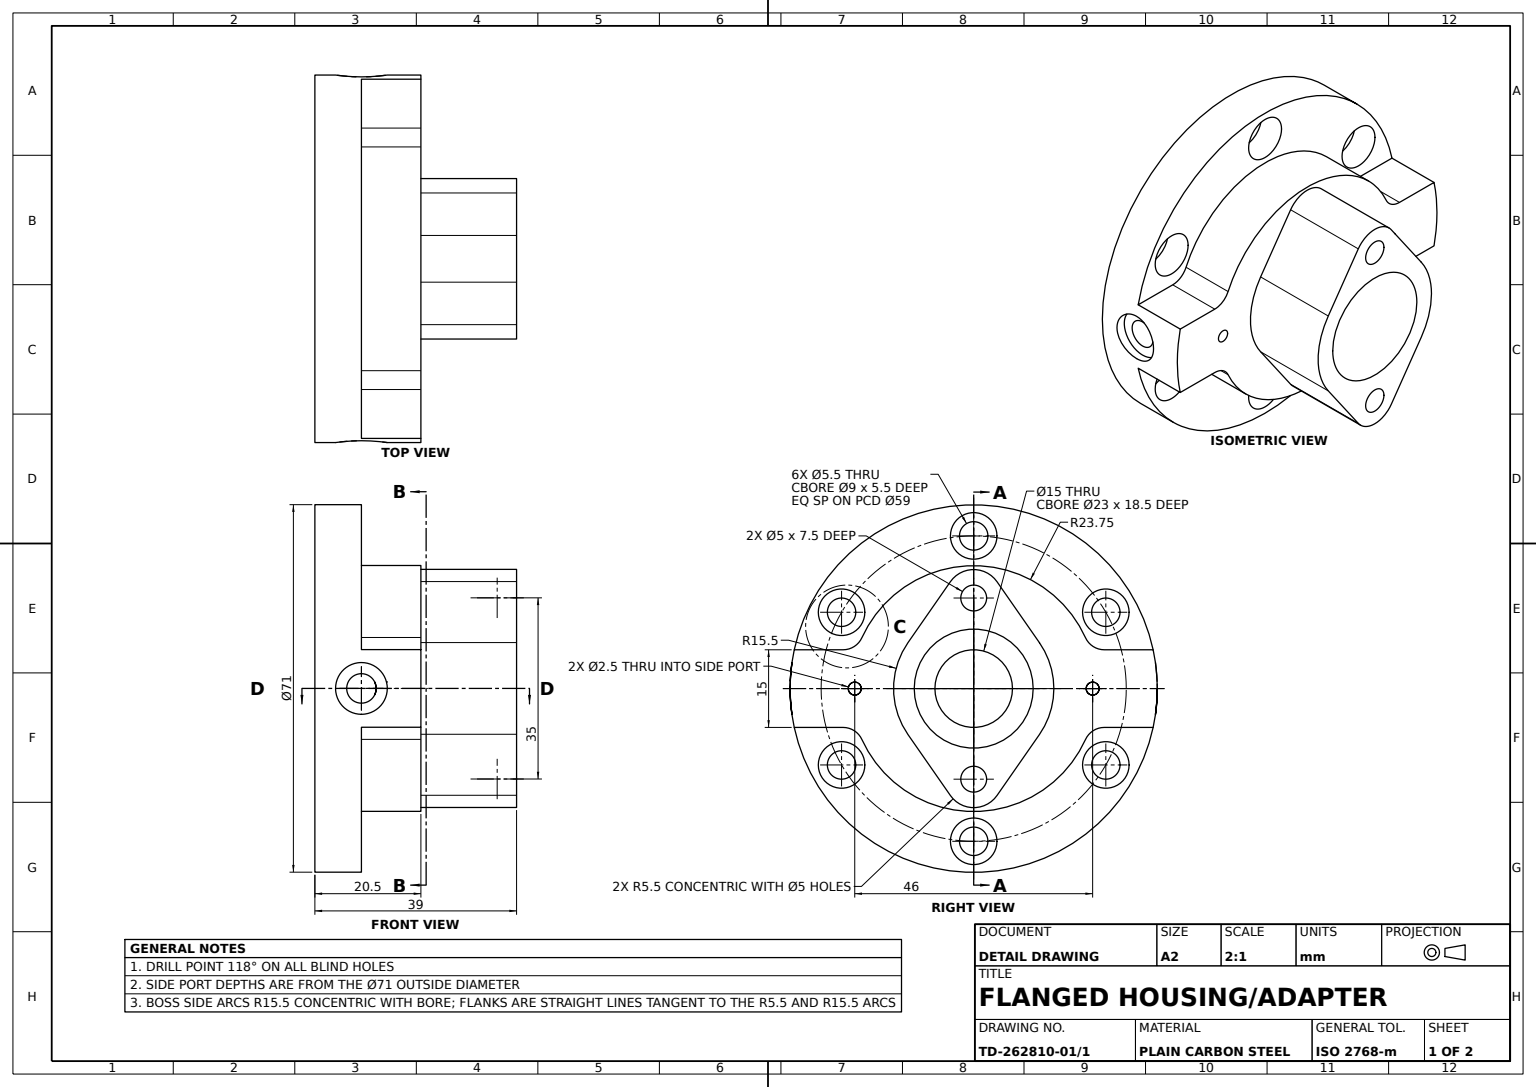
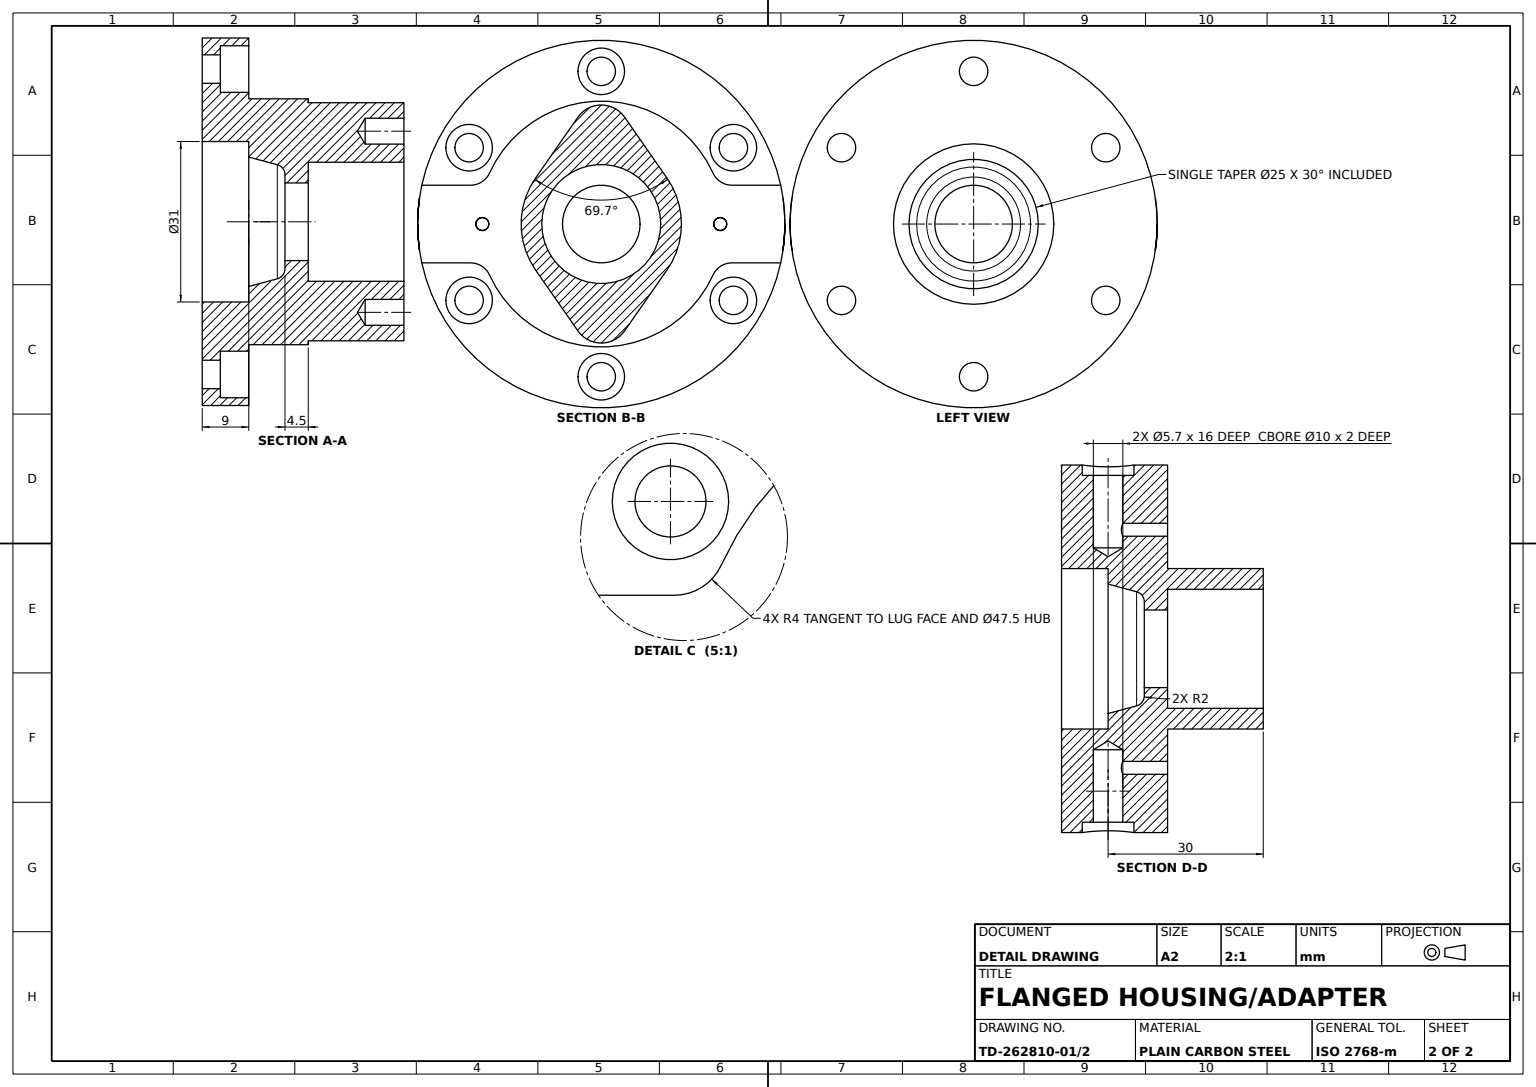
SolidWorks part; units mm, degrees
material "Plain Carbon Steel"
ref_plane "Front Plane" through (0, 0, 0) normal (0, 0, 1) x (1, 0, 0)
ref_plane "Top Plane" through (0, 0, 0) normal (0, 1, 0) x (1, 0, 0)
ref_plane "Right Plane" through (0, 0, 0) normal (1, 0, 0) x (0, 0, -1)
sketch "Flange Body Profile" plane through (0, 0, 0) normal (1, 0, 0) x (0, 0, -1)
  line L0 (0, 0) -> (0, 26.5052) construction
  line L1 (15.5, 0) -> (15.5, 9)
  line L2 (15.5, 9) -> (12.5, 9)
  line L3 (12.5, 9) -> (10.6244, 16)
  line L4 (10.6244, 16) -> (7.5, 16)
  line L5 (7.5, 16) -> (7.5, 20.5)
  line L6 (7.5, 20.5) -> (11.5, 20.5)
  line L7 (11.5, 20.5) -> (11.5, 39)
  line L8 (11.5, 39) -> (15.5, 39)
  line L9 (15.5, 39) -> (15.5, 9)
  line L10 (15.5, 9) -> (35.5, 9)
  line L11 (35.5, 9) -> (35.5, 0)
  line L12 (35.5, 0) -> (15.5, 0)
  dimension "D1" = 9
  dimension "D2" = 23
  dimension "D3" = 31
  dimension "D4" = 71
  dimension "D5" = 31
  dimension "D6" = 25
  dimension "D7" = 15
  dimension "D8" = 16
  dimension "D9" = 20.5
  dimension "D10" = 39
  dimension "D11" = 15
revolve "Flange Body" add sketch "Flange Body Profile" angle 360 about L0
sketch "Side Lug Profile" plane through (0, 39, 0) normal (0, 1, 0) x (1, 0, 0)
  line L0 (-17.5, 0) -> (17.5, 0) construction
  line L1 (-20.6429, 4.5136) -> (-8.8571, 12.7201)
  line L2 (20.6429, 4.5136) -> (8.8571, 12.7201)
  line L3 (20.6429, -4.5136) -> (8.8571, -12.7201)
  line L4 (-20.6429, -4.5136) -> (-8.8571, -12.7201)
  circle A0 centre (0, 0) radius 15.5 construction
  circle A1 centre (0, 0) radius 7.5 construction
  arc A2 (-8.8571, -12.7201) -> (8.8571, -12.7201) centre (0, 0) ccw
  circle A3 centre (0, 0) radius 7.5
  arc A4 (20.6429, -4.5136) -> (20.6429, 4.5136) centre (17.5, 0) ccw
  arc A5 (-20.6429, 4.5136) -> (-20.6429, -4.5136) centre (-17.5, 0) ccw
  arc A7 (8.8571, 12.7201) -> (-8.8571, 12.7201) centre (0, 0) ccw
  point P9 (0, 0)
  point P10 (0, 0)
  dimension "D2" = 11
  dimension "D1" = 35
extrude "Side Lugs" add sketch "Side Lug Profile" against normal blind 18.5
sketch "Oval Boss Profile" plane through (0, 9, 0) normal (0, 1, 0) x (1, 0, 0)
  line L0 (0, 35.5) -> (0, -35.5) construction
  line L1 (7.5, -34.6987) -> (7.5, -22.5347)
  line L2 (-7.5, -34.6987) -> (-7.5, -22.5347)
  line L3 (0, 0) -> (20.8022, 0) construction
  line L4 (7.5, 34.6987) -> (7.5, 22.5347)
  line L5 (-7.5, 34.6987) -> (-7.5, 22.5347)
  arc A0 (7.5, -22.5347) -> (7.5, 22.5347) centre (0, 0) ccw
  circle A1 centre (0, 0) radius 35.5 construction
  arc A2 (-7.5, -34.6987) -> (7.5, -34.6987) centre (0, 0) ccw
  arc A3 (-7.5, 34.6987) -> (7.5, 34.6987) centre (0, 0) cw
  arc A4 (-7.5, 22.5347) -> (-7.5, -22.5347) centre (0, 0) ccw
  dimension "D1" = 47.5
  dimension "D2" = 15
extrude "Oval Mounting Boss" add sketch "Oval Boss Profile" along normal up to surface (11.5 mm away) up to face at (17, 20.5, 0)
fillet "Boss Edge Fillet R4" radius 4 4 edges at (7.5, 14.75, -22.5347) (-7.5, 14.75, -22.5347) (-7.5, 14.75, 22.5347) (7.5, 14.75, 22.5347)
hole_wizard "Flange Holes 6x C'bore Ø5.5" positions "Sketch7" profile "Sketch8" legacy
sketch "Sketch7" plane through (0, 9, 0) normal (0, 1, 0) x (1, 0, 0)
  circle A0 centre (0, 0) radius 29.5 construction
  point P5 (-29.5, 0)
  point P11 (-14.75, 25.5477)
  point P12 (14.75, 25.5477)
  point P13 (29.5, 0)
  point P14 (14.75, -25.5477)
  point P15 (-14.75, -25.5477)
  dimension "D1" = 59
  dimension "D2" = 6
sketch "Sketch8" plane through (-14.75, 9, 25.5477) normal (1, 0, 0) x (0, 0, 1)
  line L0 (0, 0) -> (0, 9)
  line L1 (0, 9) -> (2.75, 9)
  line L2 (2.75, 9) -> (2.75, 5.5)
  line L3 (2.75, 5.5) -> (4.5, 5.5)
  line L4 (4.5, 5.5) -> (4.5, 0)
  line L5 (4.5, 0) -> (0, 0)
  line L6 (0, 110) -> (0, -10) construction
  dimension "Diameter" = 5.5
  dimension "Depth" = 9
  dimension "C-Bore Diameter" = 9
  dimension "C-Bore Depth" = 5.5
hole_wizard "Side Port C'bore Ø5.7" positions "3DSketch4" profile "Sketch13" legacy
sketch3d "3DSketch4"
  point P0 (0, 9, 35.5)
  point P9 (0, 9, -35.5)
sketch "Sketch13" plane through (0, 9, 35.5) normal (1, 0, 0) x (0, -1, 0)
  line L0 (0, 0) -> (0, 17.7125)
  line L1 (0, 17.7125) -> (2.85, 16)
  line L2 (2.85, 16) -> (2.85, 2)
  line L3 (2.85, 2) -> (5, 2)
  line L4 (5, 0) -> (0, 0)
  line L5 (0, -11.3109) -> (0, 121.1557) construction
  line L6 (0, 17.7125) -> (-2.85, 16) construction
  line L7 (5, 2) -> (5, 0)
  dimension "Depth" = 16
  dimension "Drill Angle" = 118
  dimension "Diameter" = 5.7
  dimension "C-Bore Diameter" = 10
  dimension "C-Bore Depth" = 2
sketch "Relief Cut Profile" plane through (0, 20.5, 0) normal (0, 1, 0) x (1, 0, 0)
  line L0 (0, 23) -> (0, -23) construction
  circle A0 centre (0, 23) radius 1.25
  circle A1 centre (0, -23) radius 1.25
  point P4 (0, 0)
  dimension "D2" = 2.5
  dimension "D1" = 46
extrude "Relief Cut" cut sketch "Relief Cut Profile" against normal up to next
hole_wizard "Lug Drill Holes Ø5" positions "Sketch15" profile "Sketch16" legacy
sketch "Sketch15" plane through (0, 39, 0) normal (0, 1, 0) x (1, 0, 0)
  point P0 (-17.5, 0)
  point P3 (17.5, 0)
sketch "Sketch16" plane through (-17.5, 39, 0) normal (1, 0, 0) x (0, 0, 1)
  line L0 (0, 0) -> (0, 9.0022)
  line L1 (0, 9.0022) -> (2.5, 7.5)
  line L2 (2.5, 7.5) -> (2.5, 0)
  line L4 (2.5, 0) -> (0, 0)
  line L6 (0, 9.0022) -> (-2.5, 7.5) construction
  line L7 (0, -4.2442) -> (0, 117.3081) construction
  dimension "Diameter" = 5
  dimension "Depth" = 7.5
  dimension "Drill Angle" = 118
sketch "Central Bore Profile" plane through (0, 0, 0) normal (1, 0, 0) x (0, 0, -1)
  line L0 (0, 0) -> (0, 26.5052) construction
  line L2 (21.6146, 9) -> (-21.6146, 9) construction
  line L4 (10.6244, 16) -> (7.5, 16) construction
  line L5 (12.5, 9) -> (10.6244, 16) construction
  line L6 (0, 0) -> (0, 39) construction
  line L7 (11.5, 20.5) -> (11.5, 39) construction
  line L8 (12.5, 9) -> (0, 9)
  line L10 (10.6244, 16) -> (7.5, 16)
  line L11 (12.5, 9) -> (10.6244, 16)
  line L14 (7.5, 20.5) -> (7.5, 16)
  line L15 (7.5, 20.5) -> (11.5, 20.5) construction
  line L16 (11.5, 20.5) -> (11.5, 39)
  line L17 (7.5, 20.5) -> (11.5, 20.5)
  line L18 (7.5, 39) -> (-7.5, 39) construction
  line L19 (11.5, 39) -> (0, 39)
  line L20 (0, 9) -> (0, 39)
revolve "Central Bore" cut sketch "Central Bore Profile" angle 360 about L6
fillet "Bore Edge Fillet R2" radius 2 1 edges at (0, 16, -10.6244)
